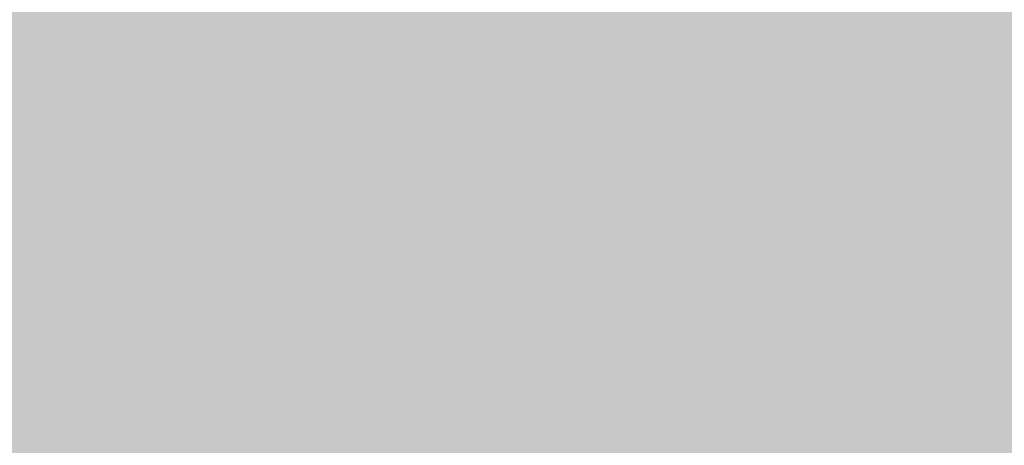
# Model space of a CAD drawing. Units: millimetres. Extents: x -22994 to 29398, y -19990 to 20176.
# Tile 78 of 135: x 226.355 to 227.437, y 84.732 to 85.199. Entities that reach past the tile are written whole.
import ezdxf
from ezdxf import colors
from ezdxf.entities.mleader import LeaderData, LeaderLine
from ezdxf.math import Vec2, Vec3

# ---------------------------------------------------------------- set-up
doc = ezdxf.new("R2010")
doc.units = ezdxf.units.MM
doc.header["$MEASUREMENT"] = 0
doc.layers.add('M-ANNO-TEXT', color=7, linetype='Continuous', lineweight=25)
doc.layers.add('M-DIMS', color=2, linetype='Continuous', lineweight=18)
doc.styles.get("Standard").update_dxf_attribs({"font": 'arial.ttf'})
doc.dimstyles.get("Standard").update_dxf_attribs({"dimtxt": 0.18, "dimasz": 10000, "dimexe": 0.18, "dimexo": 0.0625, "dimgap": 0.09, "dimtad": 0, "dimtih": 1, "dimtoh": 1, "dimdec": 0, "dimzin": 0, "dimdsep": 46, "dimtxsty": 'Standard', "dimcen": 0.09, "dimadec": 0, "dimazin": 0, "dimtfac": 1, "dimtdec": 0, "dimtofl": 0, "dimtmove": 0, "dimatfit": 3, "dimfxl": 1, "dimtolj": 1, "dimtzin": 0, "dimlwd": 30, "dimarcsym": 0})

# ---------------------------------------------------------------- blocks, each defined once
blk = doc.blocks.new('*D2')
at = {"layer": 'Defpoints', "color": 0, "transparency": 16777216}
for p in [(6.6773, 10.2713), (290.852, 10.2713), (290.852, -5.0787)]:
    blk.add_point(p, dxfattribs=at)
at = {"layer": 'M-DIMS', "color": 0, "lineweight": -2, "transparency": 16777216}
for p, q in [((6.6773, 10.2088), (6.6773, -5.2587)), ((290.852, 10.2088), (290.852, -5.2587))]:
    blk.add_line(p, q, dxfattribs=at)
at = {"layer": 'M-DIMS', "color": 0, "lineweight": 30, "transparency": 16777216}
for p, q in [((-9993.3227, -5.0787), (-19993.3227, -5.0787)), ((10290.852, -5.0787), (20290.852, -5.0787))]:
    blk.add_line(p, q, dxfattribs=at)
at = {"layer": 'M-DIMS', "color": 0, "transparency": 16777216}
for points in [[(-9993.3227, 1661.5879), (-9993.3227, -1671.7454), (6.6773, -5.0787)], [(10290.852, 1661.5879), (10290.852, -1671.7454), (290.852, -5.0787)]]:
    blk.add_solid(points, dxfattribs=at)
at = {"layer": 'M-DIMS', "color": 0, "transparency": 16777216, "insert": (148.7647, -5.0787), "char_height": 0.18, "attachment_point": 5}
blk.add_mtext('\\A1;284.2', dxfattribs=at)
blk = doc.blocks.new('*D3')
at = {"layer": 'Defpoints', "color": 0, "transparency": 16777216}
for p in [(110.2647, 204.1654), (110.2647, 176.3662), (95.8327, 127.967)]:
    blk.add_point(p, dxfattribs=at)
at = {"layer": 'M-DIMS', "color": 0, "lineweight": -2, "transparency": 16777216}
for p, q in [((95.8327, 128.0295), (95.8327, 204.3454)), ((110.2647, 176.4287), (110.2647, 204.3454))]:
    blk.add_line(p, q, dxfattribs=at)
at = {"layer": 'M-DIMS', "color": 0, "lineweight": 30, "transparency": 16777216}
for p, q in [((-9904.1673, 204.1654), (-19904.1673, 204.1654)), ((10110.2647, 204.1654), (20110.2647, 204.1654))]:
    blk.add_line(p, q, dxfattribs=at)
at = {"layer": 'M-DIMS', "color": 0, "transparency": 16777216}
for points in [[(-9904.1673, 1870.8321), (-9904.1673, -1462.5013), (95.8327, 204.1654)], [(10110.2647, 1870.8321), (10110.2647, -1462.5013), (110.2647, 204.1654)]]:
    blk.add_solid(points, dxfattribs=at)
at = {"layer": 'M-DIMS', "color": 0, "transparency": 16777216, "insert": (103.0487, 204.1654), "char_height": 0.18, "attachment_point": 5}
blk.add_mtext('\\A1;14.432', dxfattribs=at)
blk = doc.blocks.new('*D4')
at = {"layer": 'Defpoints', "color": 0, "transparency": 16777216}
for p in [(116.2647, 204.1654), (110.2647, 176.3662), (116.2647, 176.3662)]:
    blk.add_point(p, dxfattribs=at)
at = {"layer": 'M-DIMS', "color": 0, "lineweight": -2, "transparency": 16777216}
for p, q in [((110.2647, 176.4287), (110.2647, 204.3454)), ((116.2647, 176.4287), (116.2647, 204.3454))]:
    blk.add_line(p, q, dxfattribs=at)
at = {"layer": 'M-DIMS', "color": 0, "lineweight": 30, "transparency": 16777216}
for p, q in [((-9889.7353, 204.1654), (-19889.7353, 204.1654)), ((10116.2647, 204.1654), (20116.2647, 204.1654))]:
    blk.add_line(p, q, dxfattribs=at)
at = {"layer": 'M-DIMS', "color": 0, "transparency": 16777216}
for points in [[(-9889.7353, 1870.8321), (-9889.7353, -1462.5013), (110.2647, 204.1654)], [(10116.2647, 1870.8321), (10116.2647, -1462.5013), (116.2647, 204.1654)]]:
    blk.add_solid(points, dxfattribs=at)
at = {"layer": 'M-DIMS', "color": 0, "transparency": 16777216, "insert": (113.2647, 204.1654), "char_height": 0.18, "attachment_point": 5}
blk.add_mtext('\\A1;6', dxfattribs=at)
blk = doc.blocks.new('*D5')
at = {"layer": 'Defpoints', "color": 0, "transparency": 16777216}
for p in [(181.2647, 204.1654), (116.2647, 176.3662), (181.2647, 176.3662)]:
    blk.add_point(p, dxfattribs=at)
at = {"layer": 'M-DIMS', "color": 0, "lineweight": -2, "transparency": 16777216}
for p, q in [((116.2647, 176.4287), (116.2647, 204.3454)), ((181.2647, 176.4287), (181.2647, 204.3454))]:
    blk.add_line(p, q, dxfattribs=at)
at = {"layer": 'M-DIMS', "color": 0, "lineweight": 30, "transparency": 16777216}
for p, q in [((-9883.7353, 204.1654), (-19883.7353, 204.1654)), ((10181.2647, 204.1654), (20181.2647, 204.1654))]:
    blk.add_line(p, q, dxfattribs=at)
at = {"layer": 'M-DIMS', "color": 0, "transparency": 16777216}
for points in [[(-9883.7353, 1870.8321), (-9883.7353, -1462.5013), (116.2647, 204.1654)], [(10181.2647, 1870.8321), (10181.2647, -1462.5013), (181.2647, 204.1654)]]:
    blk.add_solid(points, dxfattribs=at)
at = {"layer": 'M-DIMS', "color": 0, "transparency": 16777216, "insert": (148.7647, 204.1654), "char_height": 0.18, "attachment_point": 5}
blk.add_mtext('\\A1;65', dxfattribs=at)
blk = doc.blocks.new('*D6')
at = {"layer": 'Defpoints', "color": 0, "transparency": 16777216}
for p in [(187.2647, 204.1654), (181.2647, 176.3662), (187.2647, 176.3662)]:
    blk.add_point(p, dxfattribs=at)
at = {"layer": 'M-DIMS', "color": 0, "lineweight": -2, "transparency": 16777216}
for p, q in [((181.2647, 176.4287), (181.2647, 204.3454)), ((187.2647, 176.4287), (187.2647, 204.3454))]:
    blk.add_line(p, q, dxfattribs=at)
at = {"layer": 'M-DIMS', "color": 0, "lineweight": 30, "transparency": 16777216}
for p, q in [((-9818.7353, 204.1654), (-19818.7353, 204.1654)), ((10187.2647, 204.1654), (20187.2647, 204.1654))]:
    blk.add_line(p, q, dxfattribs=at)
at = {"layer": 'M-DIMS', "color": 0, "transparency": 16777216}
for points in [[(-9818.7353, 1870.8321), (-9818.7353, -1462.5013), (181.2647, 204.1654)], [(10187.2647, 1870.8321), (10187.2647, -1462.5013), (187.2647, 204.1654)]]:
    blk.add_solid(points, dxfattribs=at)
at = {"layer": 'M-DIMS', "color": 0, "transparency": 16777216, "insert": (184.2647, 204.1654), "char_height": 0.18, "attachment_point": 5}
blk.add_mtext('\\A1;6', dxfattribs=at)
blk = doc.blocks.new('*D7')
at = {"layer": 'Defpoints', "color": 0, "transparency": 16777216}
for p in [(201.6967, 204.1654), (187.2647, 176.3662), (201.6967, 127.967)]:
    blk.add_point(p, dxfattribs=at)
at = {"layer": 'M-DIMS', "color": 0, "lineweight": -2, "transparency": 16777216}
for p, q in [((187.2647, 176.4287), (187.2647, 204.3454)), ((201.6967, 128.0295), (201.6967, 204.3454))]:
    blk.add_line(p, q, dxfattribs=at)
at = {"layer": 'M-DIMS', "color": 0, "lineweight": 30, "transparency": 16777216}
for p, q in [((-9812.7353, 204.1654), (-19812.7353, 204.1654)), ((10201.6967, 204.1654), (20201.6967, 204.1654))]:
    blk.add_line(p, q, dxfattribs=at)
at = {"layer": 'M-DIMS', "color": 0, "transparency": 16777216}
for points in [[(-9812.7353, 1870.8321), (-9812.7353, -1462.5013), (187.2647, 204.1654)], [(10201.6967, 1870.8321), (10201.6967, -1462.5013), (201.6967, 204.1654)]]:
    blk.add_solid(points, dxfattribs=at)
at = {"layer": 'M-DIMS', "color": 0, "transparency": 16777216, "insert": (194.4807, 204.1654), "char_height": 0.18, "attachment_point": 5}
blk.add_mtext('\\A1;14.432', dxfattribs=at)
blk = doc.blocks.new('*D8')
at = {"layer": 'Defpoints', "color": 0, "transparency": 16777216}
for p in [(227.6485, 204.1654), (227.6485, 146.7296), (201.6967, 127.967)]:
    blk.add_point(p, dxfattribs=at)
at = {"layer": 'M-DIMS', "color": 0, "lineweight": -2, "transparency": 16777216}
for p, q in [((201.6967, 128.0295), (201.6967, 204.3454)), ((227.6485, 146.7921), (227.6485, 204.3454))]:
    blk.add_line(p, q, dxfattribs=at)
at = {"layer": 'M-DIMS', "color": 0, "lineweight": 30, "transparency": 16777216}
for p, q in [((-9798.3033, 204.1654), (-19798.3033, 204.1654)), ((10227.6485, 204.1654), (20227.6485, 204.1654))]:
    blk.add_line(p, q, dxfattribs=at)
at = {"layer": 'M-DIMS', "color": 0, "transparency": 16777216}
for points in [[(-9798.3033, 1870.8321), (-9798.3033, -1462.5013), (201.6967, 204.1654)], [(10227.6485, 1870.8321), (10227.6485, -1462.5013), (227.6485, 204.1654)]]:
    blk.add_solid(points, dxfattribs=at)
at = {"layer": 'M-DIMS', "color": 0, "transparency": 16777216, "insert": (214.6726, 204.1654), "char_height": 0.18, "attachment_point": 5}
blk.add_mtext('\\A1;25.95', dxfattribs=at)
blk = doc.blocks.new('*D9')
at = {"layer": 'Defpoints', "color": 0, "transparency": 16777216}
for p in [(187.2647, 176.3662), (306.202, 176.3662), (290.852, 10.2713)]:
    blk.add_point(p, dxfattribs=at)
at = {"layer": 'M-DIMS', "color": 0, "lineweight": 30, "transparency": 16777216}
for p, q in [((306.202, 10176.3662), (306.202, 20176.3662)), ((306.202, -9989.7287), (306.202, -19989.7287))]:
    blk.add_line(p, q, dxfattribs=at)
at = {"layer": 'M-DIMS', "color": 0, "lineweight": -2, "transparency": 16777216}
for p, q in [((187.3272, 176.3662), (306.382, 176.3662)), ((290.9145, 10.2713), (306.382, 10.2713))]:
    blk.add_line(p, q, dxfattribs=at)
at = {"layer": 'M-DIMS', "color": 0, "transparency": 16777216}
for points in [[(-1360.4646, 10176.3662), (1972.8687, 10176.3662), (306.202, 176.3662)], [(-1360.4646, -9989.7287), (1972.8687, -9989.7287), (306.202, 10.2713)]]:
    blk.add_solid(points, dxfattribs=at)
at = {"layer": 'M-DIMS', "color": 0, "transparency": 16777216, "insert": (306.202, 93.3187), "char_height": 0.18, "attachment_point": 5}
blk.add_mtext('\\A1;166.1', dxfattribs=at)
blk = doc.blocks.new('*D10')
at = {"layer": 'Defpoints', "color": 0, "transparency": 16777216}
for p in [(125.6498, 136.0713), (133.3459, 136.0713), (133.3459, -5.0787)]:
    blk.add_point(p, dxfattribs=at)
at = {"layer": 'M-DIMS', "color": 0, "lineweight": -2, "transparency": 16777216}
for p, q in [((125.6498, 136.0088), (125.6498, -5.2587)), ((133.3459, 136.0088), (133.3459, -5.2587))]:
    blk.add_line(p, q, dxfattribs=at)
at = {"layer": 'M-DIMS', "color": 0, "lineweight": 30, "transparency": 16777216}
for p, q in [((-9874.3502, -5.0787), (-19874.3502, -5.0787)), ((10133.3459, -5.0787), (20133.3459, -5.0787))]:
    blk.add_line(p, q, dxfattribs=at)
at = {"layer": 'M-DIMS', "color": 0, "transparency": 16777216}
for points in [[(-9874.3502, 1661.5879), (-9874.3502, -1671.7454), (125.6498, -5.0787)], [(10133.3459, 1661.5879), (10133.3459, -1671.7454), (133.3459, -5.0787)]]:
    blk.add_solid(points, dxfattribs=at)
at = {"layer": 'M-DIMS', "color": 0, "transparency": 16777216, "insert": (129.4978, -5.0787), "char_height": 0.18, "attachment_point": 5}
blk.add_mtext('\\A1;7.696', dxfattribs=at)
blk = doc.blocks.new('*D11')
at = {"layer": 'Defpoints', "color": 0, "transparency": 16777216}
for p in [(133.3459, 136.0713), (135.6498, 136.0713), (135.6498, -5.0787)]:
    blk.add_point(p, dxfattribs=at)
at = {"layer": 'M-DIMS', "color": 0, "lineweight": -2, "transparency": 16777216}
for p, q in [((133.3459, 136.0088), (133.3459, -5.2587)), ((135.6498, 136.0088), (135.6498, -5.2587))]:
    blk.add_line(p, q, dxfattribs=at)
at = {"layer": 'M-DIMS', "color": 0, "lineweight": 30, "transparency": 16777216}
for p, q in [((-9866.6541, -5.0787), (-19866.6541, -5.0787)), ((10135.6498, -5.0787), (20135.6498, -5.0787))]:
    blk.add_line(p, q, dxfattribs=at)
at = {"layer": 'M-DIMS', "color": 0, "transparency": 16777216}
for points in [[(-9866.6541, 1661.5879), (-9866.6541, -1671.7454), (133.3459, -5.0787)], [(10135.6498, 1661.5879), (10135.6498, -1671.7454), (135.6498, -5.0787)]]:
    blk.add_solid(points, dxfattribs=at)
at = {"layer": 'M-DIMS', "color": 0, "transparency": 16777216, "insert": (134.4978, -5.0787), "char_height": 0.18, "attachment_point": 5}
blk.add_mtext('\\A1;2.304', dxfattribs=at)
blk = doc.blocks.new('*D12')
at = {"layer": 'Defpoints', "color": 0, "transparency": 16777216}
for p in [(135.6498, 136.0713), (145.6498, 136.0713), (145.6498, -5.0787)]:
    blk.add_point(p, dxfattribs=at)
at = {"layer": 'M-DIMS', "color": 0, "lineweight": -2, "transparency": 16777216}
for p, q in [((135.6498, 136.0088), (135.6498, -5.2587)), ((145.6498, 136.0088), (145.6498, -5.2587))]:
    blk.add_line(p, q, dxfattribs=at)
at = {"layer": 'M-DIMS', "color": 0, "lineweight": 30, "transparency": 16777216}
for p, q in [((-9864.3502, -5.0787), (-19864.3502, -5.0787)), ((10145.6498, -5.0787), (20145.6498, -5.0787))]:
    blk.add_line(p, q, dxfattribs=at)
at = {"layer": 'M-DIMS', "color": 0, "transparency": 16777216}
for points in [[(-9864.3502, 1661.5879), (-9864.3502, -1671.7454), (135.6498, -5.0787)], [(10145.6498, 1661.5879), (10145.6498, -1671.7454), (145.6498, -5.0787)]]:
    blk.add_solid(points, dxfattribs=at)
at = {"layer": 'M-DIMS', "color": 0, "transparency": 16777216, "insert": (140.6498, -5.0787), "char_height": 0.18, "attachment_point": 5}
blk.add_mtext('\\A1;10', dxfattribs=at)
blk = doc.blocks.new('*D13')
at = {"layer": 'Defpoints', "color": 0, "transparency": 16777216}
for p in [(145.6498, 136.0713), (155.6498, 136.0713), (155.6498, -5.0787)]:
    blk.add_point(p, dxfattribs=at)
at = {"layer": 'M-DIMS', "color": 0, "lineweight": -2, "transparency": 16777216}
for p, q in [((145.6498, 136.0088), (145.6498, -5.2587)), ((155.6498, 136.0088), (155.6498, -5.2587))]:
    blk.add_line(p, q, dxfattribs=at)
at = {"layer": 'M-DIMS', "color": 0, "lineweight": 30, "transparency": 16777216}
for p, q in [((-9854.3502, -5.0787), (-19854.3502, -5.0787)), ((10155.6498, -5.0787), (20155.6498, -5.0787))]:
    blk.add_line(p, q, dxfattribs=at)
at = {"layer": 'M-DIMS', "color": 0, "transparency": 16777216}
for points in [[(-9854.3502, 1661.5879), (-9854.3502, -1671.7454), (145.6498, -5.0787)], [(10155.6498, 1661.5879), (10155.6498, -1671.7454), (155.6498, -5.0787)]]:
    blk.add_solid(points, dxfattribs=at)
at = {"layer": 'M-DIMS', "color": 0, "transparency": 16777216, "insert": (150.6498, -5.0787), "char_height": 0.18, "attachment_point": 5}
blk.add_mtext('\\A1;10', dxfattribs=at)
blk = doc.blocks.new('*D14')
at = {"layer": 'Defpoints', "color": 0, "transparency": 16777216}
for p in [(155.6498, 136.0713), (165.6498, 136.0713), (165.6498, -5.0787)]:
    blk.add_point(p, dxfattribs=at)
at = {"layer": 'M-DIMS', "color": 0, "lineweight": -2, "transparency": 16777216}
for p, q in [((155.6498, 136.0088), (155.6498, -5.2587)), ((165.6498, 136.0088), (165.6498, -5.2587))]:
    blk.add_line(p, q, dxfattribs=at)
at = {"layer": 'M-DIMS', "color": 0, "lineweight": 30, "transparency": 16777216}
for p, q in [((-9844.3502, -5.0787), (-19844.3502, -5.0787)), ((10165.6498, -5.0787), (20165.6498, -5.0787))]:
    blk.add_line(p, q, dxfattribs=at)
at = {"layer": 'M-DIMS', "color": 0, "transparency": 16777216}
for points in [[(-9844.3502, 1661.5879), (-9844.3502, -1671.7454), (155.6498, -5.0787)], [(10165.6498, 1661.5879), (10165.6498, -1671.7454), (165.6498, -5.0787)]]:
    blk.add_solid(points, dxfattribs=at)
at = {"layer": 'M-DIMS', "color": 0, "transparency": 16777216, "insert": (160.6498, -5.0787), "char_height": 0.18, "attachment_point": 5}
blk.add_mtext('\\A1;10', dxfattribs=at)
blk = doc.blocks.new('*D15')
at = {"layer": 'Defpoints', "color": 0, "transparency": 16777216}
for p in [(173.3459, 154.788), (173.3459, 136.0713), (306.202, 136.0713)]:
    blk.add_point(p, dxfattribs=at)
at = {"layer": 'M-DIMS', "color": 0, "lineweight": 30, "transparency": 16777216}
for p, q in [((306.202, 10154.788), (306.202, 20154.788)), ((306.202, -9863.9287), (306.202, -19863.9287))]:
    blk.add_line(p, q, dxfattribs=at)
at = {"layer": 'M-DIMS', "color": 0, "lineweight": -2, "transparency": 16777216}
for p, q in [((173.4084, 154.788), (306.382, 154.788)), ((173.4084, 136.0713), (306.382, 136.0713))]:
    blk.add_line(p, q, dxfattribs=at)
at = {"layer": 'M-DIMS', "color": 0, "transparency": 16777216}
for points in [[(-1360.4646, 10154.788), (1972.8687, 10154.788), (306.202, 154.788)], [(-1360.4646, -9863.9287), (1972.8687, -9863.9287), (306.202, 136.0713)]]:
    blk.add_solid(points, dxfattribs=at)
at = {"layer": 'M-DIMS', "color": 0, "transparency": 16777216, "insert": (306.202, 145.4297), "char_height": 0.18, "attachment_point": 5}
blk.add_mtext('\\A1;18.717', dxfattribs=at)
blk = doc.blocks.new('*D16')
at = {"layer": 'Defpoints', "color": 0, "transparency": 16777216}
for p in [(120.1702, 204.1654), (110.4658, 48.0349), (120.1702, 48.0349)]:
    blk.add_point(p, dxfattribs=at)
at = {"layer": 'M-DIMS', "color": 0, "lineweight": -2, "transparency": 16777216}
for p, q in [((110.4658, 48.0974), (110.4658, 204.3454)), ((120.1702, 48.0974), (120.1702, 204.3454))]:
    blk.add_line(p, q, dxfattribs=at)
at = {"layer": 'M-DIMS', "color": 0, "lineweight": 30, "transparency": 16777216}
for p, q in [((-9889.5342, 204.1654), (-19889.5342, 204.1654)), ((10120.1702, 204.1654), (20120.1702, 204.1654))]:
    blk.add_line(p, q, dxfattribs=at)
at = {"layer": 'M-DIMS', "color": 0, "transparency": 16777216}
for points in [[(-9889.5342, 1870.8321), (-9889.5342, -1462.5013), (110.4658, 204.1654)], [(10120.1702, 1870.8321), (10120.1702, -1462.5013), (120.1702, 204.1654)]]:
    blk.add_solid(points, dxfattribs=at)
at = {"layer": 'M-DIMS', "color": 0, "transparency": 16777216, "insert": (115.318, 204.1654), "char_height": 0.18, "attachment_point": 5}
blk.add_mtext('\\A1;9.704', dxfattribs=at)
blk = doc.blocks.new('*D17')
at = {"layer": 'Defpoints', "color": 0, "transparency": 16777216}
for p in [(126.1702, 204.1654), (120.1702, 48.0349), (126.1702, 48.0349)]:
    blk.add_point(p, dxfattribs=at)
at = {"layer": 'M-DIMS', "color": 0, "lineweight": -2, "transparency": 16777216}
for p, q in [((120.1702, 48.0974), (120.1702, 204.3454)), ((126.1702, 48.0974), (126.1702, 204.3454))]:
    blk.add_line(p, q, dxfattribs=at)
at = {"layer": 'M-DIMS', "color": 0, "lineweight": 30, "transparency": 16777216}
for p, q in [((-9879.8298, 204.1654), (-19879.8298, 204.1654)), ((10126.1702, 204.1654), (20126.1702, 204.1654))]:
    blk.add_line(p, q, dxfattribs=at)
at = {"layer": 'M-DIMS', "color": 0, "transparency": 16777216}
for points in [[(-9879.8298, 1870.8321), (-9879.8298, -1462.5013), (120.1702, 204.1654)], [(10126.1702, 1870.8321), (10126.1702, -1462.5013), (126.1702, 204.1654)]]:
    blk.add_solid(points, dxfattribs=at)
at = {"layer": 'M-DIMS', "color": 0, "transparency": 16777216, "insert": (123.1702, 204.1654), "char_height": 0.18, "attachment_point": 5}
blk.add_mtext('\\A1;6', dxfattribs=at)
blk = doc.blocks.new('*D18')
at = {"layer": 'Defpoints', "color": 0, "transparency": 16777216}
for p in [(132.1702, 204.1654), (126.1702, 48.0349), (132.1702, 48.0349)]:
    blk.add_point(p, dxfattribs=at)
at = {"layer": 'M-DIMS', "color": 0, "lineweight": -2, "transparency": 16777216}
for p, q in [((126.1702, 48.0974), (126.1702, 204.3454)), ((132.1702, 48.0974), (132.1702, 204.3454))]:
    blk.add_line(p, q, dxfattribs=at)
at = {"layer": 'M-DIMS', "color": 0, "lineweight": 30, "transparency": 16777216}
for p, q in [((-9873.8298, 204.1654), (-19873.8298, 204.1654)), ((10132.1702, 204.1654), (20132.1702, 204.1654))]:
    blk.add_line(p, q, dxfattribs=at)
at = {"layer": 'M-DIMS', "color": 0, "transparency": 16777216}
for points in [[(-9873.8298, 1870.8321), (-9873.8298, -1462.5013), (126.1702, 204.1654)], [(10132.1702, 1870.8321), (10132.1702, -1462.5013), (132.1702, 204.1654)]]:
    blk.add_solid(points, dxfattribs=at)
at = {"layer": 'M-DIMS', "color": 0, "transparency": 16777216, "insert": (129.1702, 204.1654), "char_height": 0.18, "attachment_point": 5}
blk.add_mtext('\\A1;6', dxfattribs=at)
blk = doc.blocks.new('*D19')
at = {"layer": 'Defpoints', "color": 0, "transparency": 16777216}
for p in [(138.1702, 204.1654), (132.1702, 48.0349), (138.1702, 48.0349)]:
    blk.add_point(p, dxfattribs=at)
at = {"layer": 'M-DIMS', "color": 0, "lineweight": -2, "transparency": 16777216}
for p, q in [((132.1702, 48.0974), (132.1702, 204.3454)), ((138.1702, 48.0974), (138.1702, 204.3454))]:
    blk.add_line(p, q, dxfattribs=at)
at = {"layer": 'M-DIMS', "color": 0, "lineweight": 30, "transparency": 16777216}
for p, q in [((-9867.8298, 204.1654), (-19867.8298, 204.1654)), ((10138.1702, 204.1654), (20138.1702, 204.1654))]:
    blk.add_line(p, q, dxfattribs=at)
at = {"layer": 'M-DIMS', "color": 0, "transparency": 16777216}
for points in [[(-9867.8298, 1870.8321), (-9867.8298, -1462.5013), (132.1702, 204.1654)], [(10138.1702, 1870.8321), (10138.1702, -1462.5013), (138.1702, 204.1654)]]:
    blk.add_solid(points, dxfattribs=at)
at = {"layer": 'M-DIMS', "color": 0, "transparency": 16777216, "insert": (135.1702, 204.1654), "char_height": 0.18, "attachment_point": 5}
blk.add_mtext('\\A1;6', dxfattribs=at)
blk = doc.blocks.new('*D20')
at = {"layer": 'Defpoints', "color": 0, "transparency": 16777216}
for p in [(144.1702, 204.1654), (138.1702, 48.0349), (144.1702, 48.0349)]:
    blk.add_point(p, dxfattribs=at)
at = {"layer": 'M-DIMS', "color": 0, "lineweight": -2, "transparency": 16777216}
for p, q in [((138.1702, 48.0974), (138.1702, 204.3454)), ((144.1702, 48.0974), (144.1702, 204.3454))]:
    blk.add_line(p, q, dxfattribs=at)
at = {"layer": 'M-DIMS', "color": 0, "lineweight": 30, "transparency": 16777216}
for p, q in [((-9861.8298, 204.1654), (-19861.8298, 204.1654)), ((10144.1702, 204.1654), (20144.1702, 204.1654))]:
    blk.add_line(p, q, dxfattribs=at)
at = {"layer": 'M-DIMS', "color": 0, "transparency": 16777216}
for points in [[(-9861.8298, 1870.8321), (-9861.8298, -1462.5013), (138.1702, 204.1654)], [(10144.1702, 1870.8321), (10144.1702, -1462.5013), (144.1702, 204.1654)]]:
    blk.add_solid(points, dxfattribs=at)
at = {"layer": 'M-DIMS', "color": 0, "transparency": 16777216, "insert": (141.1702, 204.1654), "char_height": 0.18, "attachment_point": 5}
blk.add_mtext('\\A1;6', dxfattribs=at)
blk = doc.blocks.new('*D21')
at = {"layer": 'Defpoints', "color": 0, "transparency": 16777216}
for p in [(149.1157, 204.1654), (144.1702, 48.0349), (149.1157, 48.0349)]:
    blk.add_point(p, dxfattribs=at)
at = {"layer": 'M-DIMS', "color": 0, "lineweight": -2, "transparency": 16777216}
for p, q in [((144.1702, 48.0974), (144.1702, 204.3454)), ((149.1157, 48.0974), (149.1157, 204.3454))]:
    blk.add_line(p, q, dxfattribs=at)
at = {"layer": 'M-DIMS', "color": 0, "lineweight": 30, "transparency": 16777216}
for p, q in [((-9855.8298, 204.1654), (-19855.8298, 204.1654)), ((10149.1157, 204.1654), (20149.1157, 204.1654))]:
    blk.add_line(p, q, dxfattribs=at)
at = {"layer": 'M-DIMS', "color": 0, "transparency": 16777216}
for points in [[(-9855.8298, 1870.8321), (-9855.8298, -1462.5013), (144.1702, 204.1654)], [(10149.1157, 1870.8321), (10149.1157, -1462.5013), (149.1157, 204.1654)]]:
    blk.add_solid(points, dxfattribs=at)
at = {"layer": 'M-DIMS', "color": 0, "transparency": 16777216, "insert": (146.6429, 204.1654), "char_height": 0.18, "attachment_point": 5}
blk.add_mtext('\\A1;4.945', dxfattribs=at)
blk = doc.blocks.new('*D22')
at = {"layer": 'Defpoints', "color": 0, "transparency": 16777216}
for p in [(149.1157, 30.9895), (155.1157, 30.9895), (155.1157, -5.0787)]:
    blk.add_point(p, dxfattribs=at)
at = {"layer": 'M-DIMS', "color": 0, "lineweight": -2, "transparency": 16777216}
for p, q in [((149.1157, 30.927), (149.1157, -5.2587)), ((155.1157, 30.927), (155.1157, -5.2587))]:
    blk.add_line(p, q, dxfattribs=at)
at = {"layer": 'M-DIMS', "color": 0, "lineweight": 30, "transparency": 16777216}
for p, q in [((-9850.8843, -5.0787), (-19850.8843, -5.0787)), ((10155.1157, -5.0787), (20155.1157, -5.0787))]:
    blk.add_line(p, q, dxfattribs=at)
at = {"layer": 'M-DIMS', "color": 0, "transparency": 16777216}
for points in [[(-9850.8843, 1661.5879), (-9850.8843, -1671.7454), (149.1157, -5.0787)], [(10155.1157, 1661.5879), (10155.1157, -1671.7454), (155.1157, -5.0787)]]:
    blk.add_solid(points, dxfattribs=at)
at = {"layer": 'M-DIMS', "color": 0, "transparency": 16777216, "insert": (152.1157, -5.0787), "char_height": 0.18, "attachment_point": 5}
blk.add_mtext('\\A1;6', dxfattribs=at)
blk = doc.blocks.new('*D23')
at = {"layer": 'Defpoints', "color": 0, "transparency": 16777216}
for p in [(155.1157, 30.9895), (161.1157, 30.9895), (161.1157, -5.0787)]:
    blk.add_point(p, dxfattribs=at)
at = {"layer": 'M-DIMS', "color": 0, "lineweight": -2, "transparency": 16777216}
for p, q in [((155.1157, 30.927), (155.1157, -5.2587)), ((161.1157, 30.927), (161.1157, -5.2587))]:
    blk.add_line(p, q, dxfattribs=at)
at = {"layer": 'M-DIMS', "color": 0, "lineweight": 30, "transparency": 16777216}
for p, q in [((-9844.8843, -5.0787), (-19844.8843, -5.0787)), ((10161.1157, -5.0787), (20161.1157, -5.0787))]:
    blk.add_line(p, q, dxfattribs=at)
at = {"layer": 'M-DIMS', "color": 0, "transparency": 16777216}
for points in [[(-9844.8843, 1661.5879), (-9844.8843, -1671.7454), (155.1157, -5.0787)], [(10161.1157, 1661.5879), (10161.1157, -1671.7454), (161.1157, -5.0787)]]:
    blk.add_solid(points, dxfattribs=at)
at = {"layer": 'M-DIMS', "color": 0, "transparency": 16777216, "insert": (158.1157, -5.0787), "char_height": 0.18, "attachment_point": 5}
blk.add_mtext('\\A1;6', dxfattribs=at)
blk = doc.blocks.new('*D24')
at = {"layer": 'Defpoints', "color": 0, "transparency": 16777216}
for p in [(161.1157, 30.9895), (166.4387, 30.9895), (166.4387, -5.0787)]:
    blk.add_point(p, dxfattribs=at)
at = {"layer": 'M-DIMS', "color": 0, "lineweight": -2, "transparency": 16777216}
for p, q in [((161.1157, 30.927), (161.1157, -5.2587)), ((166.4387, 30.927), (166.4387, -5.2587))]:
    blk.add_line(p, q, dxfattribs=at)
at = {"layer": 'M-DIMS', "color": 0, "lineweight": 30, "transparency": 16777216}
for p, q in [((-9838.8843, -5.0787), (-19838.8843, -5.0787)), ((10166.4387, -5.0787), (20166.4387, -5.0787))]:
    blk.add_line(p, q, dxfattribs=at)
at = {"layer": 'M-DIMS', "color": 0, "transparency": 16777216}
for points in [[(-9838.8843, 1661.5879), (-9838.8843, -1671.7454), (161.1157, -5.0787)], [(10166.4387, 1661.5879), (10166.4387, -1671.7454), (166.4387, -5.0787)]]:
    blk.add_solid(points, dxfattribs=at)
at = {"layer": 'M-DIMS', "color": 0, "transparency": 16777216, "insert": (163.7772, -5.0787), "char_height": 0.18, "attachment_point": 5}
blk.add_mtext('\\A1;5.323', dxfattribs=at)
blk = doc.blocks.new('*D25')
at = {"layer": 'Defpoints', "color": 0, "transparency": 16777216}
for p in [(166.4387, 30.9895), (172.4387, 30.9895), (172.4387, -5.0787)]:
    blk.add_point(p, dxfattribs=at)
at = {"layer": 'M-DIMS', "color": 0, "lineweight": -2, "transparency": 16777216}
for p, q in [((166.4387, 30.927), (166.4387, -5.2587)), ((172.4387, 30.927), (172.4387, -5.2587))]:
    blk.add_line(p, q, dxfattribs=at)
at = {"layer": 'M-DIMS', "color": 0, "lineweight": 30, "transparency": 16777216}
for p, q in [((-9833.5613, -5.0787), (-19833.5613, -5.0787)), ((10172.4387, -5.0787), (20172.4387, -5.0787))]:
    blk.add_line(p, q, dxfattribs=at)
at = {"layer": 'M-DIMS', "color": 0, "transparency": 16777216}
for points in [[(-9833.5613, 1661.5879), (-9833.5613, -1671.7454), (166.4387, -5.0787)], [(10172.4387, 1661.5879), (10172.4387, -1671.7454), (172.4387, -5.0787)]]:
    blk.add_solid(points, dxfattribs=at)
at = {"layer": 'M-DIMS', "color": 0, "transparency": 16777216, "insert": (169.4387, -5.0787), "char_height": 0.18, "attachment_point": 5}
blk.add_mtext('\\A1;6', dxfattribs=at)
blk = doc.blocks.new('*D26')
at = {"layer": 'Defpoints', "color": 0, "transparency": 16777216}
for p in [(172.4387, 30.9895), (178.4387, 30.9895), (178.4387, -5.0787)]:
    blk.add_point(p, dxfattribs=at)
at = {"layer": 'M-DIMS', "color": 0, "lineweight": -2, "transparency": 16777216}
for p, q in [((172.4387, 30.927), (172.4387, -5.2587)), ((178.4387, 30.927), (178.4387, -5.2587))]:
    blk.add_line(p, q, dxfattribs=at)
at = {"layer": 'M-DIMS', "color": 0, "lineweight": 30, "transparency": 16777216}
for p, q in [((-9827.5613, -5.0787), (-19827.5613, -5.0787)), ((10178.4387, -5.0787), (20178.4387, -5.0787))]:
    blk.add_line(p, q, dxfattribs=at)
at = {"layer": 'M-DIMS', "color": 0, "transparency": 16777216}
for points in [[(-9827.5613, 1661.5879), (-9827.5613, -1671.7454), (172.4387, -5.0787)], [(10178.4387, 1661.5879), (10178.4387, -1671.7454), (178.4387, -5.0787)]]:
    blk.add_solid(points, dxfattribs=at)
at = {"layer": 'M-DIMS', "color": 0, "transparency": 16777216, "insert": (175.4387, -5.0787), "char_height": 0.18, "attachment_point": 5}
blk.add_mtext('\\A1;6', dxfattribs=at)
blk = doc.blocks.new('*D27')
at = {"layer": 'Defpoints', "color": 0, "transparency": 16777216}
for p in [(178.4387, 30.9895), (188.1175, 30.9895), (188.1175, -5.0787)]:
    blk.add_point(p, dxfattribs=at)
at = {"layer": 'M-DIMS', "color": 0, "lineweight": -2, "transparency": 16777216}
for p, q in [((178.4387, 30.927), (178.4387, -5.2587)), ((188.1175, 30.927), (188.1175, -5.2587))]:
    blk.add_line(p, q, dxfattribs=at)
at = {"layer": 'M-DIMS', "color": 0, "lineweight": 30, "transparency": 16777216}
for p, q in [((-9821.5613, -5.0787), (-19821.5613, -5.0787)), ((10188.1175, -5.0787), (20188.1175, -5.0787))]:
    blk.add_line(p, q, dxfattribs=at)
at = {"layer": 'M-DIMS', "color": 0, "transparency": 16777216}
for points in [[(-9821.5613, 1661.5879), (-9821.5613, -1671.7454), (178.4387, -5.0787)], [(10188.1175, 1661.5879), (10188.1175, -1671.7454), (188.1175, -5.0787)]]:
    blk.add_solid(points, dxfattribs=at)
at = {"layer": 'M-DIMS', "color": 0, "transparency": 16777216, "insert": (183.2781, -5.0787), "char_height": 0.18, "attachment_point": 5}
blk.add_mtext('\\A1;9.679', dxfattribs=at)
blk = doc.blocks.new('*D28')
at = {"layer": 'Defpoints', "color": 0, "transparency": 16777216}
for p in [(188.1175, 48.0349), (306.202, 48.0349), (188.1175, 30.9895)]:
    blk.add_point(p, dxfattribs=at)
at = {"layer": 'M-DIMS', "color": 0, "lineweight": 30, "transparency": 16777216}
for p, q in [((306.202, 10048.0349), (306.202, 20048.0349)), ((306.202, -9969.0105), (306.202, -19969.0105))]:
    blk.add_line(p, q, dxfattribs=at)
at = {"layer": 'M-DIMS', "color": 0, "lineweight": -2, "transparency": 16777216}
for p, q in [((188.18, 48.0349), (306.382, 48.0349)), ((188.18, 30.9895), (306.382, 30.9895))]:
    blk.add_line(p, q, dxfattribs=at)
at = {"layer": 'M-DIMS', "color": 0, "transparency": 16777216}
for points in [[(-1360.4646, 10048.0349), (1972.8687, 10048.0349), (306.202, 48.0349)], [(-1360.4646, -9969.0105), (1972.8687, -9969.0105), (306.202, 30.9895)]]:
    blk.add_solid(points, dxfattribs=at)
at = {"layer": 'M-DIMS', "color": 0, "transparency": 16777216, "insert": (306.202, 39.5122), "char_height": 0.18, "attachment_point": 5}
blk.add_mtext('\\A1;17.045', dxfattribs=at)
blk = doc.blocks.new('*D29')
at = {"layer": 'Defpoints', "color": 0, "transparency": 16777216}
for p in [(36.8006, 80.045), (64.0296, 80.045)]:
    blk.add_point(p, dxfattribs=at)
at = {"layer": 'M-DIMS', "color": 0, "lineweight": -2, "transparency": 16777216}
for p, q in [((50.4151, 79.955), (50.4151, 80.135)), ((50.3251, 80.045), (50.5051, 80.045))]:
    blk.add_line(p, q, dxfattribs=at)
at = {"layer": 'M-DIMS', "color": 0, "lineweight": 30, "transparency": 16777216}
blk.add_line((20064.0296, 80.0303), (10064.0296, 80.0377), dxfattribs=at)
at = {"layer": 'M-DIMS', "color": 0, "transparency": 16777216}
blk.add_solid([(10064.0309, 1746.7043), (10064.0284, -1586.629), (64.0296, 80.045)], dxfattribs=at)
at = {"layer": 'M-DIMS', "color": 0, "transparency": 16777216, "insert": (20064.5213, 80.0303), "char_height": 0.18, "attachment_point": 5}
blk.add_mtext('\\A1;∅27.23', dxfattribs=at)
blk = doc.blocks.new('*D30')
at = {"layer": 'Defpoints', "color": 0, "transparency": 16777216}
for p in [(216.3148, 146.7291), (238.9821, 146.73)]:
    blk.add_point(p, dxfattribs=at)
at = {"layer": 'M-DIMS', "color": 0, "lineweight": 30, "transparency": 16777216}
blk.add_line((20238.9821, 147.4959), (10238.9821, 147.1129), dxfattribs=at)
at = {"layer": 'M-DIMS', "color": 0, "lineweight": -2, "transparency": 16777216}
for p, q in [((227.6485, 146.6396), (227.6485, 146.8196)), ((227.5585, 146.7296), (227.7385, 146.7296))]:
    blk.add_line(p, q, dxfattribs=at)
at = {"layer": 'M-DIMS', "color": 0, "transparency": 16777216}
blk.add_solid([(10238.9183, 1813.7796), (10239.0459, -1519.5537), (238.9821, 146.73)], dxfattribs=at)
at = {"layer": 'M-DIMS', "color": 0, "transparency": 16777216, "insert": (20239.5436, 147.4959), "char_height": 0.18, "attachment_point": 5}
blk.add_mtext('\\A1;∅22.667', dxfattribs=at)
blk = doc.blocks.new('*D31')
at = {"layer": 'Defpoints', "color": 0, "transparency": 16777216}
for p in [(223.1641, 146.7291), (232.1328, 146.73)]:
    blk.add_point(p, dxfattribs=at)
at = {"layer": 'M-DIMS', "color": 0, "lineweight": 30, "transparency": 16777216}
blk.add_line((20232.1327, 148.6656), (10232.1328, 147.6978), dxfattribs=at)
at = {"layer": 'M-DIMS', "color": 0, "lineweight": -2, "transparency": 16777216}
for p, q in [((227.6485, 146.6396), (227.6485, 146.8196)), ((227.5585, 146.7296), (227.7385, 146.7296))]:
    blk.add_line(p, q, dxfattribs=at)
at = {"layer": 'M-DIMS', "color": 0, "transparency": 16777216}
blk.add_solid([(10231.9715, 1814.3645), (10232.2941, -1518.9688), (232.1328, 146.73)], dxfattribs=at)
at = {"layer": 'M-DIMS', "color": 0, "transparency": 16777216, "insert": (20232.6245, 148.6656), "char_height": 0.18, "attachment_point": 5}
blk.add_mtext('\\A1;∅8.969', dxfattribs=at)
blk = doc.blocks.new('*D36')
at = {"layer": 'Defpoints', "color": 0, "transparency": 16777216}
for p in [(46.39, 31.3035), (46.3875, 26.5934)]:
    blk.add_point(p, dxfattribs=at)
at = {"layer": 'M-DIMS', "color": 0, "lineweight": 30, "transparency": 16777216}
for p, q in [((57.1499, 20031.3006), (51.77, 10031.302)), ((10057.1499, 20031.3006), (57.1499, 20031.3006))]:
    blk.add_line(p, q, dxfattribs=at)
at = {"layer": 'M-DIMS', "color": 0, "lineweight": -2, "transparency": 16777216}
for p, q in [((46.3887, 28.8585), (46.3887, 29.0385)), ((46.2987, 28.9485), (46.4787, 28.9485))]:
    blk.add_line(p, q, dxfattribs=at)
at = {"layer": 'M-DIMS', "color": 0, "transparency": 16777216}
blk.add_solid([(-1614.8965, 10032.1987), (1718.4364, 10030.4054), (46.39, 31.3035)], dxfattribs=at)
at = {"layer": 'M-DIMS', "color": 0, "transparency": 16777216, "insert": (10057.5542, 20031.3006), "char_height": 0.18, "attachment_point": 5}
blk.add_mtext('\\A1;∅4.71', dxfattribs=at)
blk = doc.blocks.new('*D37')
at = {"layer": 'Defpoints', "color": 0, "transparency": 16777216}
for p in [(54.8343, 118.6145), (59.4936, 118.614)]:
    blk.add_point(p, dxfattribs=at)
at = {"layer": 'M-DIMS', "color": 0, "lineweight": -2, "transparency": 16777216}
for p, q in [((57.1639, 118.5243), (57.1639, 118.7043)), ((57.0739, 118.6143), (57.2539, 118.6143))]:
    blk.add_line(p, q, dxfattribs=at)
at = {"layer": 'M-DIMS', "color": 0, "lineweight": 30, "transparency": 16777216}
blk.add_line((20059.4934, 116.2531), (10059.4935, 117.4336), dxfattribs=at)
at = {"layer": 'M-DIMS', "color": 0, "transparency": 16777216}
blk.add_solid([(10059.6902, 1784.1002), (10059.2968, -1549.2331), (59.4936, 118.614)], dxfattribs=at)
at = {"layer": 'M-DIMS', "color": 0, "transparency": 16777216, "insert": (20059.9852, 116.2531), "char_height": 0.18, "attachment_point": 5}
blk.add_mtext('\\A1;∅4.659', dxfattribs=at)

msp = doc.modelspace()

# ---------------------------------------------------------------- dimensions: what is measured, and where the dimension line sits
at = {"layer": 'M-DIMS'}
for base, p1, p2, override, picture, middle in [((306.202, 176.3662), (290.852, 10.2713), (187.2647, 176.3662), {"dimdec": 1, "dimlfac": 1, "dimrnd": 0, "dimzin": 0, "dimdsep": 46, "dimlunit": 2}, '*D9', (306.202, 93.3187)), ((306.202, 136.0713), (173.3459, 154.788), (173.3459, 136.0713), {"dimdec": 3, "dimlfac": 1, "dimrnd": 0, "dimzin": 0, "dimdsep": 46, "dimlunit": 2}, '*D15', (306.202, 145.4297)), ((306.202, 48.0349), (188.1175, 30.9895), (188.1175, 48.0349), {"dimdec": 3, "dimlfac": 1, "dimrnd": 0, "dimzin": 0, "dimdsep": 46, "dimlunit": 2}, '*D28', (306.202, 39.5122))]:
    dim = msp.add_linear_dim(base=base, p1=p1, p2=p2, angle=90, dimstyle='Standard', override=override, dxfattribs=at)
    dim.commit()
    dim.dimension.update_dxf_attribs({"geometry": picture, "text_midpoint": middle})
for p1, p2, override, picture, middle in [((46.3875, 26.5934), (46.39, 31.3035), {"dimdec": 2, "dimlfac": 1, "dimrnd": 0, "dimzin": 0, "dimdsep": 46, "dimlunit": 2}, '*D36', (10057.5542, 20031.3006)), ((223.1641, 146.7291), (232.1328, 146.73), {"dimdec": 3, "dimlfac": 1, "dimrnd": 0, "dimzin": 0, "dimdsep": 46, "dimlunit": 2}, '*D31', (20232.1327, 148.6656)), ((216.3148, 146.7291), (238.9821, 146.73), {"dimdec": 3, "dimlfac": 1, "dimrnd": 0, "dimzin": 0, "dimdsep": 46, "dimlunit": 2}, '*D30', (20238.9821, 147.4959))]:
    dim = msp.add_diameter_dim_2p(p1=p1, p2=p2, dimstyle='Standard', override=override, dxfattribs=at)
    dim.commit()
    dim.dimension.update_dxf_attribs({"geometry": picture, "text_midpoint": middle, "dimtype": 163})
for base, p1, p2, override, picture, middle in [((110.2647, 204.1654), (95.8327, 127.967), (110.2647, 176.3662), {"dimdec": 3, "dimlfac": 1, "dimrnd": 0, "dimzin": 0, "dimdsep": 46, "dimlunit": 2}, '*D3', (103.0487, 204.1654)), ((116.2647, 204.1654), (110.2647, 176.3662), (116.2647, 176.3662), {"dimdec": 0, "dimlfac": 1, "dimrnd": 0, "dimzin": 0, "dimdsep": 46, "dimlunit": 2}, '*D4', (113.2647, 204.1654)), ((120.1702, 204.1654), (110.4658, 48.0349), (120.1702, 48.0349), {"dimdec": 3, "dimlfac": 1, "dimrnd": 0, "dimzin": 0, "dimdsep": 46, "dimlunit": 2}, '*D16', (115.318, 204.1654)), ((181.2647, 204.1654), (116.2647, 176.3662), (181.2647, 176.3662), {"dimdec": 0, "dimlfac": 1, "dimrnd": 0, "dimzin": 0, "dimdsep": 46, "dimlunit": 2}, '*D5', (148.7647, 204.1654)), ((126.1702, 204.1654), (120.1702, 48.0349), (126.1702, 48.0349), {"dimdec": 0, "dimlfac": 1, "dimrnd": 0, "dimzin": 0, "dimdsep": 46, "dimlunit": 2}, '*D17', (123.1702, 204.1654)), ((132.1702, 204.1654), (126.1702, 48.0349), (132.1702, 48.0349), {"dimdec": 0, "dimlfac": 1, "dimrnd": 0, "dimzin": 0, "dimdsep": 46, "dimlunit": 2}, '*D18', (129.1702, 204.1654)), ((138.1702, 204.1654), (132.1702, 48.0349), (138.1702, 48.0349), {"dimdec": 0, "dimlfac": 1, "dimrnd": 0, "dimzin": 0, "dimdsep": 46, "dimlunit": 2}, '*D19', (135.1702, 204.1654)), ((144.1702, 204.1654), (138.1702, 48.0349), (144.1702, 48.0349), {"dimdec": 0, "dimlfac": 1, "dimrnd": 0, "dimzin": 0, "dimdsep": 46, "dimlunit": 2}, '*D20', (141.1702, 204.1654)), ((149.11567, 204.16539), (144.17023, 48.03494), (149.11567, 48.03494), {"dimdec": 3, "dimlfac": 1, "dimrnd": 0, "dimzin": 0, "dimdsep": 46, "dimlunit": 2}, '*D21', (146.64295, 204.16539)), ((187.2647, 204.1654), (181.2647, 176.3662), (187.2647, 176.3662), {"dimdec": 0, "dimlfac": 1, "dimrnd": 0, "dimzin": 0, "dimdsep": 46, "dimlunit": 2}, '*D6', (184.2647, 204.1654)), ((201.6967, 204.1654), (187.2647, 176.3662), (201.6967, 127.967), {"dimdec": 3, "dimlfac": 1, "dimrnd": 0, "dimzin": 0, "dimdsep": 46, "dimlunit": 2}, '*D7', (194.4807, 204.1654)), ((227.6485, 204.1654), (201.6967, 127.967), (227.6485, 146.7296), {"dimdec": 2, "dimlfac": 1, "dimrnd": 0, "dimzin": 0, "dimdsep": 46, "dimlunit": 2}, '*D8', (214.6726, 204.1654)), ((290.852, -5.0787), (6.6773, 10.2713), (290.852, 10.2713), {"dimdec": 1, "dimlfac": 1, "dimrnd": 0, "dimzin": 0, "dimdsep": 46, "dimlunit": 2}, '*D2', (148.7647, -5.0787)), ((133.3459, -5.0787), (125.6498, 136.0713), (133.3459, 136.0713), {"dimdec": 3, "dimlfac": 1, "dimrnd": 0, "dimzin": 0, "dimdsep": 46, "dimlunit": 2}, '*D10', (129.4978, -5.0787)), ((135.6498, -5.0787), (133.3459, 136.0713), (135.6498, 136.0713), {"dimdec": 3, "dimlfac": 1, "dimrnd": 0, "dimzin": 0, "dimdsep": 46, "dimlunit": 2}, '*D11', (134.4978, -5.0787)), ((145.6498, -5.0787), (135.6498, 136.0713), (145.6498, 136.0713), {"dimdec": 0, "dimlfac": 1, "dimrnd": 0, "dimzin": 0, "dimdsep": 46, "dimlunit": 2}, '*D12', (140.6498, -5.0787)), ((155.6498, -5.0787), (145.6498, 136.0713), (155.6498, 136.0713), {"dimdec": 0, "dimlfac": 1, "dimrnd": 0, "dimzin": 0, "dimdsep": 46, "dimlunit": 2}, '*D13', (150.6498, -5.0787)), ((155.1157, -5.0787), (149.1157, 30.9895), (155.1157, 30.9895), {"dimdec": 0, "dimlfac": 1, "dimrnd": 0, "dimzin": 0, "dimdsep": 46, "dimlunit": 2}, '*D22', (152.1157, -5.0787)), ((161.1157, -5.0787), (155.1157, 30.9895), (161.1157, 30.9895), {"dimdec": 0, "dimlfac": 1, "dimrnd": 0, "dimzin": 0, "dimdsep": 46, "dimlunit": 2}, '*D23', (158.1157, -5.0787)), ((165.6498, -5.0787), (155.6498, 136.0713), (165.6498, 136.0713), {"dimdec": 0, "dimlfac": 1, "dimrnd": 0, "dimzin": 0, "dimdsep": 46, "dimlunit": 2}, '*D14', (160.6498, -5.0787)), ((166.4387, -5.0787), (161.1157, 30.9895), (166.4387, 30.9895), {"dimdec": 3, "dimlfac": 1, "dimrnd": 0, "dimzin": 0, "dimdsep": 46, "dimlunit": 2}, '*D24', (163.7772, -5.0787)), ((172.4387, -5.0787), (166.4387, 30.9895), (172.4387, 30.9895), {"dimdec": 0, "dimlfac": 1, "dimrnd": 0, "dimzin": 0, "dimdsep": 46, "dimlunit": 2}, '*D25', (169.4387, -5.0787)), ((178.4387, -5.0787), (172.4387, 30.9895), (178.4387, 30.9895), {"dimdec": 0, "dimlfac": 1, "dimrnd": 0, "dimzin": 0, "dimdsep": 46, "dimlunit": 2}, '*D26', (175.4387, -5.0787)), ((188.1175, -5.0787), (178.4387, 30.9895), (188.1175, 30.9895), {"dimdec": 3, "dimlfac": 1, "dimrnd": 0, "dimzin": 0, "dimdsep": 46, "dimlunit": 2}, '*D27', (183.2781, -5.0787))]:
    dim = msp.add_linear_dim(base=base, p1=p1, p2=p2, dimstyle='Standard', override=override, dxfattribs=at)
    dim.commit()
    dim.dimension.update_dxf_attribs({"geometry": picture, "text_midpoint": middle})
for p1, p2, override, picture, middle in [((54.8343, 118.6145), (59.4936, 118.614), {"dimdec": 3, "dimlfac": 1, "dimrnd": 0, "dimzin": 0, "dimdsep": 46, "dimlunit": 2}, '*D37', (20059.4934, 116.2531)), ((36.8006, 80.045), (64.0296, 80.045), {"dimdec": 2, "dimlfac": 1, "dimrnd": 0, "dimzin": 0, "dimdsep": 46, "dimlunit": 2}, '*D29', (20064.0296, 80.0303))]:
    dim = msp.add_diameter_dim_2p(p1=p1, p2=p2, dimstyle='Standard', override=override, dxfattribs=at)
    dim.commit()
    dim.dimension.update_dxf_attribs({"geometry": picture, "text_midpoint": middle})

# ---------------------------------------------------------------- leaders
at = {"layer": 'M-ANNO-TEXT'}
ml = msp.add_multileader_mtext('Standard', dxfattribs=at)
ml.set_content('combustion chamber', color=256)
ml.set_leader_properties()
ml.build(insert=Vec2(0, 0))
ml.multileader.update_dxf_attribs({"dogleg_length": 0.36, "arrow_head_size": 200})
ctx = ml.context
ctx.base_point, ctx.char_height, ctx.arrow_head_size, ctx.landing_gap_size, ctx.plane_origin = Vec3(215.7321, 57.9149), 3, 200, 0.09, Vec3(189.1175, 57.9149)
notes = []
notes.append((ctx, [(0, (1, 1, 0), (215.3721, 57.9149), (1, 0), 0.36, [(0, [(189.1175, 57.9149)], 0, [])])]))
ctx.mtext.insert, ctx.mtext.flow_direction = Vec3(215.8221, 59.4394), 5
for ctx, leaders in notes:
    for number, flags, end, landing, length, lines in leaders:
        leader = LeaderData()
        leader.index, (leader.has_last_leader_line, leader.has_dogleg_vector, leader.attachment_direction) = number, flags
        leader.last_leader_point, leader.dogleg_vector, leader.dogleg_length = Vec3(end), Vec3(landing), length
        for number, points, colour, breaks in lines:
            line = LeaderLine()
            line.index, line.vertices, line.color, line.breaks = number, Vec3.list(points), colors.encode_raw_color(colour), breaks
            leader.lines.append(line)
        ctx.leaders.append(leader)

doc.saveas('drawing.dxf')
